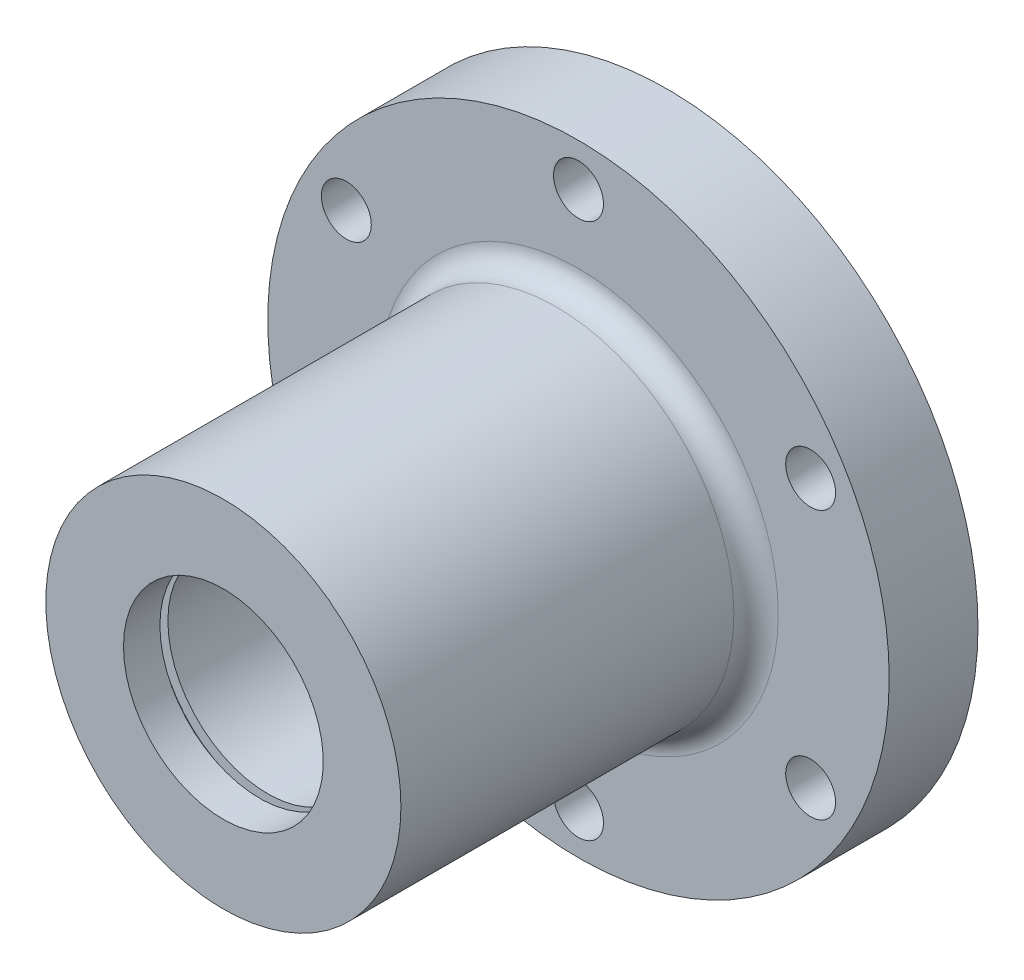
ISO-10303-21;
HEADER;
FILE_DESCRIPTION(('STEP AP214'),'2;1');
FILE_NAME('part.step','',(''),(''),'','','');
FILE_SCHEMA(('AUTOMOTIVE_DESIGN { 1 0 10303 214 1 1 1 1 }'));
ENDSEC;
DATA;
#1=APPLICATION_CONTEXT('core data for automotive mechanical design processes');
#2=APPLICATION_PROTOCOL_DEFINITION('international standard','automotive_design',2000,#1);
#3=PRODUCT_CONTEXT('',#1,'mechanical');
#4=PRODUCT('Part','Part','',(#3));
#5=PRODUCT_RELATED_PRODUCT_CATEGORY('part','',(#4));
#6=PRODUCT_DEFINITION_FORMATION('','',#4);
#7=PRODUCT_DEFINITION_CONTEXT('part definition',#1,'design');
#8=PRODUCT_DEFINITION('design','',#6,#7);
#9=PRODUCT_DEFINITION_SHAPE('','',#8);
#10=(LENGTH_UNIT() NAMED_UNIT(*) SI_UNIT(.MILLI.,.METRE.));
#11=(NAMED_UNIT(*) PLANE_ANGLE_UNIT() SI_UNIT($,.RADIAN.));
#12=(NAMED_UNIT(*) SI_UNIT($,.STERADIAN.) SOLID_ANGLE_UNIT());
#13=UNCERTAINTY_MEASURE_WITH_UNIT(LENGTH_MEASURE(1.E-05),#10,'distance_accuracy_value','');
#14=(GEOMETRIC_REPRESENTATION_CONTEXT(3) GLOBAL_UNCERTAINTY_ASSIGNED_CONTEXT((#13)) GLOBAL_UNIT_ASSIGNED_CONTEXT((#10,
#11,#12)) REPRESENTATION_CONTEXT('',''));
#15=CARTESIAN_POINT('',(0.,0.,0.));
#16=DIRECTION('',(0.,0.,1.));
#17=DIRECTION('',(1.,0.,0.));
#18=AXIS2_PLACEMENT_3D('',#15,#16,#17);
#19=CARTESIAN_POINT('',(0.,0.,12.7));
#20=DIRECTION('',(0.,0.,-1.));
#21=DIRECTION('',(-1.,0.,0.));
#22=AXIS2_PLACEMENT_3D('',#19,#20,#21);
#23=CYLINDRICAL_SURFACE('',#22,44.45);
#24=CARTESIAN_POINT('',(0.,0.,12.7));
#25=DIRECTION('',(0.,0.,1.));
#26=DIRECTION('',(1.,0.,0.));
#27=AXIS2_PLACEMENT_3D('',#24,#25,#26);
#28=CIRCLE('',#27,44.45);
#29=CARTESIAN_POINT('',(44.45,0.,12.7));
#30=VERTEX_POINT('',#29);
#31=EDGE_CURVE('E48',#30,#30,#28,.T.);
#32=ORIENTED_EDGE('',*,*,#31,.F.);
#33=EDGE_LOOP('',(#32));
#34=FACE_BOUND('',#33,.T.);
#35=CARTESIAN_POINT('',(0.,0.,0.));
#36=DIRECTION('',(0.,0.,1.));
#37=DIRECTION('',(1.,0.,0.));
#38=AXIS2_PLACEMENT_3D('',#35,#36,#37);
#39=CIRCLE('',#38,44.45);
#40=CARTESIAN_POINT('',(44.45,0.,0.));
#41=VERTEX_POINT('',#40);
#42=EDGE_CURVE('E55',#41,#41,#39,.T.);
#43=ORIENTED_EDGE('',*,*,#42,.T.);
#44=EDGE_LOOP('',(#43));
#45=FACE_BOUND('',#44,.T.);
#46=ADVANCED_FACE('F40',(#34,#45),#23,.T.);
#47=CARTESIAN_POINT('',(0.,0.,12.7));
#48=DIRECTION('',(0.,0.,1.));
#49=DIRECTION('',(1.,0.,0.));
#50=AXIS2_PLACEMENT_3D('',#47,#48,#49);
#51=PLANE('',#50);
#52=CARTESIAN_POINT('',(0.,0.,12.7));
#53=DIRECTION('',(0.,0.,1.));
#54=DIRECTION('',(1.,0.,0.));
#55=AXIS2_PLACEMENT_3D('',#52,#53,#54);
#56=CIRCLE('',#55,28.575);
#57=CARTESIAN_POINT('',(28.575,0.,12.7));
#58=VERTEX_POINT('',#57);
#59=EDGE_CURVE('E10',#58,#58,#56,.F.);
#60=ORIENTED_EDGE('',*,*,#59,.T.);
#61=EDGE_LOOP('',(#60));
#62=FACE_BOUND('',#61,.T.);
#63=CARTESIAN_POINT('',(-1.25238909962569E-12,38.3450832342934,12.7));
#64=DIRECTION('',(0.,0.,1.));
#65=DIRECTION('',(1.,0.,0.));
#66=AXIS2_PLACEMENT_3D('',#63,#64,#65);
#67=CIRCLE('',#66,3.5687);
#68=CARTESIAN_POINT('',(3.56869999999875,38.3450832342934,12.7));
#69=VERTEX_POINT('',#68);
#70=EDGE_CURVE('E54',#69,#69,#67,.T.);
#71=ORIENTED_EDGE('',*,*,#70,.F.);
#72=EDGE_LOOP('',(#71));
#73=FACE_BOUND('',#72,.T.);
#74=CARTESIAN_POINT('',(33.2078161911255,19.1725416171468,12.7));
#75=DIRECTION('',(0.,0.,1.));
#76=DIRECTION('',(1.,0.,0.));
#77=AXIS2_PLACEMENT_3D('',#74,#75,#76);
#78=CIRCLE('',#77,3.56870000000124);
#79=CARTESIAN_POINT('',(36.7765161911268,19.1725416171468,12.7));
#80=VERTEX_POINT('',#79);
#81=EDGE_CURVE('E56',#80,#80,#78,.T.);
#82=ORIENTED_EDGE('',*,*,#81,.F.);
#83=EDGE_LOOP('',(#82));
#84=FACE_BOUND('',#83,.T.);
#85=CARTESIAN_POINT('',(33.2078161911255,-19.1725416171465,12.7));
#86=DIRECTION('',(0.,0.,1.));
#87=DIRECTION('',(1.,0.,0.));
#88=AXIS2_PLACEMENT_3D('',#85,#86,#87);
#89=CIRCLE('',#88,3.56870000000238);
#90=CARTESIAN_POINT('',(36.7765161911279,-19.1725416171465,12.7));
#91=VERTEX_POINT('',#90);
#92=EDGE_CURVE('E65',#91,#91,#89,.T.);
#93=ORIENTED_EDGE('',*,*,#92,.F.);
#94=EDGE_LOOP('',(#93));
#95=FACE_BOUND('',#94,.T.);
#96=CARTESIAN_POINT('',(-1.20231643282915E-12,-38.3450832342931,12.7));
#97=DIRECTION('',(0.,0.,1.));
#98=DIRECTION('',(1.,0.,0.));
#99=AXIS2_PLACEMENT_3D('',#96,#97,#98);
#100=CIRCLE('',#99,3.56870000000269);
#101=CARTESIAN_POINT('',(3.56870000000149,-38.3450832342931,12.7));
#102=VERTEX_POINT('',#101);
#103=EDGE_CURVE('E61',#102,#102,#100,.T.);
#104=ORIENTED_EDGE('',*,*,#103,.F.);
#105=EDGE_LOOP('',(#104));
#106=FACE_BOUND('',#105,.T.);
#107=CARTESIAN_POINT('',(-33.207816191128,-19.1725416171465,12.7));
#108=DIRECTION('',(0.,0.,1.));
#109=DIRECTION('',(1.,0.,0.));
#110=AXIS2_PLACEMENT_3D('',#107,#108,#109);
#111=CIRCLE('',#110,3.56870000000184);
#112=CARTESIAN_POINT('',(-29.6391161911261,-19.1725416171465,12.7));
#113=VERTEX_POINT('',#112);
#114=EDGE_CURVE('E67',#113,#113,#111,.T.);
#115=ORIENTED_EDGE('',*,*,#114,.F.);
#116=EDGE_LOOP('',(#115));
#117=FACE_BOUND('',#116,.T.);
#118=CARTESIAN_POINT('',(-33.207816191128,19.1725416171468,12.7));
#119=DIRECTION('',(0.,0.,1.));
#120=DIRECTION('',(1.,0.,0.));
#121=AXIS2_PLACEMENT_3D('',#118,#119,#120);
#122=CIRCLE('',#121,3.56870000000052);
#123=CARTESIAN_POINT('',(-29.6391161911275,19.1725416171468,12.7));
#124=VERTEX_POINT('',#123);
#125=EDGE_CURVE('E72',#124,#124,#122,.T.);
#126=ORIENTED_EDGE('',*,*,#125,.F.);
#127=EDGE_LOOP('',(#126));
#128=FACE_BOUND('',#127,.T.);
#129=ORIENTED_EDGE('',*,*,#31,.T.);
#130=EDGE_LOOP('',(#129));
#131=FACE_BOUND('',#130,.T.);
#132=ADVANCED_FACE('F189',(#62,#73,#84,#95,#106,#117,#128,#131),#51,.T.);
#133=CARTESIAN_POINT('',(0.,0.,0.));
#134=DIRECTION('',(0.,0.,1.));
#135=DIRECTION('',(1.,0.,0.));
#136=AXIS2_PLACEMENT_3D('',#133,#134,#135);
#137=PLANE('',#136);
#138=CARTESIAN_POINT('',(-1.25238909962569E-12,38.3450832342934,0.));
#139=DIRECTION('',(0.,0.,-1.));
#140=DIRECTION('',(-1.,0.,0.));
#141=AXIS2_PLACEMENT_3D('',#138,#139,#140);
#142=CIRCLE('',#141,5.15619999999839);
#143=CARTESIAN_POINT('',(-5.15619999999964,38.3450832342934,0.));
#144=VERTEX_POINT('',#143);
#145=EDGE_CURVE('E142',#144,#144,#142,.T.);
#146=ORIENTED_EDGE('',*,*,#145,.F.);
#147=EDGE_LOOP('',(#146));
#148=FACE_BOUND('',#147,.T.);
#149=CARTESIAN_POINT('',(33.2078161911254,19.1725416171464,0.));
#150=DIRECTION('',(0.,0.,-1.));
#151=DIRECTION('',(-1.,0.,0.));
#152=AXIS2_PLACEMENT_3D('',#149,#150,#151);
#153=CIRCLE('',#152,5.1562);
#154=CARTESIAN_POINT('',(28.0516161911254,19.1725416171464,0.));
#155=VERTEX_POINT('',#154);
#156=EDGE_CURVE('E123',#155,#155,#153,.T.);
#157=ORIENTED_EDGE('',*,*,#156,.F.);
#158=EDGE_LOOP('',(#157));
#159=FACE_BOUND('',#158,.T.);
#160=CARTESIAN_POINT('',(33.2078161911251,-19.1725416171471,0.));
#161=DIRECTION('',(0.,0.,-1.));
#162=DIRECTION('',(-1.,0.,0.));
#163=AXIS2_PLACEMENT_3D('',#160,#161,#162);
#164=CIRCLE('',#163,5.15620000000149);
#165=CARTESIAN_POINT('',(28.0516161911236,-19.1725416171471,0.));
#166=VERTEX_POINT('',#165);
#167=EDGE_CURVE('E116',#166,#166,#164,.T.);
#168=ORIENTED_EDGE('',*,*,#167,.F.);
#169=EDGE_LOOP('',(#168));
#170=FACE_BOUND('',#169,.T.);
#171=CARTESIAN_POINT('',(-2.00302158664965E-12,-38.3450832342934,0.));
#172=DIRECTION('',(0.,0.,-1.));
#173=DIRECTION('',(-1.,0.,0.));
#174=AXIS2_PLACEMENT_3D('',#171,#172,#173);
#175=CIRCLE('',#174,5.15620000000176);
#176=CARTESIAN_POINT('',(-5.15620000000376,-38.3450832342934,0.));
#177=VERTEX_POINT('',#176);
#178=EDGE_CURVE('E130',#177,#177,#175,.T.);
#179=ORIENTED_EDGE('',*,*,#178,.F.);
#180=EDGE_LOOP('',(#179));
#181=FACE_BOUND('',#180,.T.);
#182=CARTESIAN_POINT('',(-33.2078161911287,-19.1725416171464,0.));
#183=DIRECTION('',(0.,0.,-1.));
#184=DIRECTION('',(-1.,0.,0.));
#185=AXIS2_PLACEMENT_3D('',#182,#183,#184);
#186=CIRCLE('',#185,5.15620000000049);
#187=CARTESIAN_POINT('',(-38.3640161911292,-19.1725416171464,0.));
#188=VERTEX_POINT('',#187);
#189=EDGE_CURVE('E133',#188,#188,#186,.T.);
#190=ORIENTED_EDGE('',*,*,#189,.F.);
#191=EDGE_LOOP('',(#190));
#192=FACE_BOUND('',#191,.T.);
#193=CARTESIAN_POINT('',(-33.2078161911283,19.172541617147,0.));
#194=DIRECTION('',(0.,0.,-1.));
#195=DIRECTION('',(-1.,0.,0.));
#196=AXIS2_PLACEMENT_3D('',#193,#194,#195);
#197=CIRCLE('',#196,5.15619999999885);
#198=CARTESIAN_POINT('',(-38.3640161911271,19.172541617147,0.));
#199=VERTEX_POINT('',#198);
#200=EDGE_CURVE('E140',#199,#199,#197,.T.);
#201=ORIENTED_EDGE('',*,*,#200,.F.);
#202=EDGE_LOOP('',(#201));
#203=FACE_BOUND('',#202,.T.);
#204=CARTESIAN_POINT('',(0.,0.,0.));
#205=DIRECTION('',(0.,0.,-1.));
#206=DIRECTION('',(-1.,0.,0.));
#207=AXIS2_PLACEMENT_3D('',#204,#205,#206);
#208=CIRCLE('',#207,20.6375);
#209=CARTESIAN_POINT('',(-20.6375,0.,0.));
#210=VERTEX_POINT('',#209);
#211=EDGE_CURVE('E83',#210,#210,#208,.T.);
#212=ORIENTED_EDGE('',*,*,#211,.F.);
#213=EDGE_LOOP('',(#212));
#214=FACE_BOUND('',#213,.T.);
#215=ORIENTED_EDGE('',*,*,#42,.F.);
#216=EDGE_LOOP('',(#215));
#217=FACE_BOUND('',#216,.T.);
#218=ADVANCED_FACE('F183',(#148,#159,#170,#181,#192,#203,#214,#217),#137,.F.);
#219=CARTESIAN_POINT('',(0.,0.,63.5));
#220=DIRECTION('',(0.,0.,-1.));
#221=DIRECTION('',(-1.,0.,0.));
#222=AXIS2_PLACEMENT_3D('',#219,#220,#221);
#223=CYLINDRICAL_SURFACE('',#222,25.4);
#224=CARTESIAN_POINT('',(0.,0.,15.875));
#225=DIRECTION('',(0.,0.,1.));
#226=DIRECTION('',(1.,0.,0.));
#227=AXIS2_PLACEMENT_3D('',#224,#225,#226);
#228=CIRCLE('',#227,25.4);
#229=CARTESIAN_POINT('',(25.4,0.,15.875));
#230=VERTEX_POINT('',#229);
#231=EDGE_CURVE('E42',#230,#230,#228,.T.);
#232=ORIENTED_EDGE('',*,*,#231,.T.);
#233=EDGE_LOOP('',(#232));
#234=FACE_BOUND('',#233,.T.);
#235=CARTESIAN_POINT('',(0.,0.,63.5));
#236=DIRECTION('',(0.,0.,1.));
#237=DIRECTION('',(1.,0.,0.));
#238=AXIS2_PLACEMENT_3D('',#235,#236,#237);
#239=CIRCLE('',#238,25.4);
#240=CARTESIAN_POINT('',(25.4,0.,63.5));
#241=VERTEX_POINT('',#240);
#242=EDGE_CURVE('E77',#241,#241,#239,.T.);
#243=ORIENTED_EDGE('',*,*,#242,.F.);
#244=EDGE_LOOP('',(#243));
#245=FACE_BOUND('',#244,.T.);
#246=ADVANCED_FACE('F188',(#234,#245),#223,.T.);
#247=CARTESIAN_POINT('',(0.,0.,63.5));
#248=DIRECTION('',(0.,0.,1.));
#249=DIRECTION('',(1.,0.,0.));
#250=AXIS2_PLACEMENT_3D('',#247,#248,#249);
#251=PLANE('',#250);
#252=CARTESIAN_POINT('',(0.,0.,63.5));
#253=DIRECTION('',(0.,0.,-1.));
#254=DIRECTION('',(-1.,0.,0.));
#255=AXIS2_PLACEMENT_3D('',#252,#253,#254);
#256=CIRCLE('',#255,14.2875);
#257=CARTESIAN_POINT('',(-14.2875,0.,63.5));
#258=VERTEX_POINT('',#257);
#259=EDGE_CURVE('E107',#258,#258,#256,.T.);
#260=ORIENTED_EDGE('',*,*,#259,.T.);
#261=EDGE_LOOP('',(#260));
#262=FACE_BOUND('',#261,.T.);
#263=ORIENTED_EDGE('',*,*,#242,.T.);
#264=EDGE_LOOP('',(#263));
#265=FACE_BOUND('',#264,.T.);
#266=ADVANCED_FACE('F216',(#262,#265),#251,.T.);
#267=CARTESIAN_POINT('',(0.,0.,6.35));
#268=DIRECTION('',(0.,0.,-1.));
#269=DIRECTION('',(-1.,0.,0.));
#270=AXIS2_PLACEMENT_3D('',#267,#268,#269);
#271=CYLINDRICAL_SURFACE('',#270,20.6375);
#272=CARTESIAN_POINT('',(0.,0.,6.35));
#273=DIRECTION('',(0.,0.,-1.));
#274=DIRECTION('',(-1.,0.,0.));
#275=AXIS2_PLACEMENT_3D('',#272,#273,#274);
#276=CIRCLE('',#275,20.6375);
#277=CARTESIAN_POINT('',(-20.6375,0.,6.35));
#278=VERTEX_POINT('',#277);
#279=EDGE_CURVE('E76',#278,#278,#276,.T.);
#280=ORIENTED_EDGE('',*,*,#279,.F.);
#281=EDGE_LOOP('',(#280));
#282=FACE_BOUND('',#281,.T.);
#283=ORIENTED_EDGE('',*,*,#211,.T.);
#284=EDGE_LOOP('',(#283));
#285=FACE_BOUND('',#284,.T.);
#286=ADVANCED_FACE('F218',(#282,#285),#271,.F.);
#287=CARTESIAN_POINT('',(0.,0.,6.35));
#288=DIRECTION('',(0.,0.,-1.));
#289=DIRECTION('',(-1.,0.,0.));
#290=AXIS2_PLACEMENT_3D('',#287,#288,#289);
#291=PLANE('',#290);
#292=CARTESIAN_POINT('',(0.,0.,6.35));
#293=DIRECTION('',(0.,0.,-1.));
#294=DIRECTION('',(-1.,0.,0.));
#295=AXIS2_PLACEMENT_3D('',#292,#293,#294);
#296=CIRCLE('',#295,9.525);
#297=CARTESIAN_POINT('',(-9.525,0.,6.35));
#298=VERTEX_POINT('',#297);
#299=EDGE_CURVE('E85',#298,#298,#296,.T.);
#300=ORIENTED_EDGE('',*,*,#299,.F.);
#301=EDGE_LOOP('',(#300));
#302=FACE_BOUND('',#301,.T.);
#303=ORIENTED_EDGE('',*,*,#279,.T.);
#304=EDGE_LOOP('',(#303));
#305=FACE_BOUND('',#304,.T.);
#306=ADVANCED_FACE('F225',(#302,#305),#291,.T.);
#307=CARTESIAN_POINT('',(0.,0.,15.875));
#308=DIRECTION('',(0.,0.,-1.));
#309=DIRECTION('',(-1.,0.,0.));
#310=AXIS2_PLACEMENT_3D('',#307,#308,#309);
#311=CYLINDRICAL_SURFACE('',#310,9.525);
#312=CARTESIAN_POINT('',(0.,0.,15.875));
#313=DIRECTION('',(0.,0.,-1.));
#314=DIRECTION('',(-1.,0.,0.));
#315=AXIS2_PLACEMENT_3D('',#312,#313,#314);
#316=CIRCLE('',#315,9.525);
#317=CARTESIAN_POINT('',(-9.525,0.,15.875));
#318=VERTEX_POINT('',#317);
#319=EDGE_CURVE('E90',#318,#318,#316,.T.);
#320=CARTESIAN_POINT('',(-9.525,0.,15.875));
#321=CARTESIAN_POINT('',(-9.525,0.,15.77578125));
#322=CARTESIAN_POINT('',(-9.525,0.,15.6765625));
#323=CARTESIAN_POINT('',(-9.525,0.,15.478125));
#324=CARTESIAN_POINT('',(-9.525,0.,15.37890625));
#325=CARTESIAN_POINT('',(-9.525,0.,15.18046875));
#326=CARTESIAN_POINT('',(-9.525,0.,15.08125));
#327=CARTESIAN_POINT('',(-9.525,0.,14.8828125));
#328=CARTESIAN_POINT('',(-9.525,0.,14.78359375));
#329=CARTESIAN_POINT('',(-9.525,0.,14.58515625));
#330=CARTESIAN_POINT('',(-9.525,0.,14.4859375));
#331=CARTESIAN_POINT('',(-9.525,0.,14.2875));
#332=CARTESIAN_POINT('',(-9.525,0.,14.18828125));
#333=CARTESIAN_POINT('',(-9.525,0.,13.98984375));
#334=CARTESIAN_POINT('',(-9.525,0.,13.890625));
#335=CARTESIAN_POINT('',(-9.525,0.,13.6921875));
#336=CARTESIAN_POINT('',(-9.525,0.,13.59296875));
#337=CARTESIAN_POINT('',(-9.525,0.,13.39453125));
#338=CARTESIAN_POINT('',(-9.525,0.,13.2953125));
#339=CARTESIAN_POINT('',(-9.525,0.,13.096875));
#340=CARTESIAN_POINT('',(-9.525,0.,12.99765625));
#341=CARTESIAN_POINT('',(-9.525,0.,12.79921875));
#342=CARTESIAN_POINT('',(-9.525,0.,12.7));
#343=CARTESIAN_POINT('',(-9.525,0.,12.5015625));
#344=CARTESIAN_POINT('',(-9.525,0.,12.40234375));
#345=CARTESIAN_POINT('',(-9.525,0.,12.20390625));
#346=CARTESIAN_POINT('',(-9.525,0.,12.1046875));
#347=CARTESIAN_POINT('',(-9.525,0.,11.90625));
#348=CARTESIAN_POINT('',(-9.525,0.,11.80703125));
#349=CARTESIAN_POINT('',(-9.525,0.,11.60859375));
#350=CARTESIAN_POINT('',(-9.525,0.,11.509375));
#351=CARTESIAN_POINT('',(-9.525,0.,11.3109375));
#352=CARTESIAN_POINT('',(-9.525,0.,11.21171875));
#353=CARTESIAN_POINT('',(-9.525,0.,11.01328125));
#354=CARTESIAN_POINT('',(-9.525,0.,10.9140625));
#355=CARTESIAN_POINT('',(-9.525,0.,10.715625));
#356=CARTESIAN_POINT('',(-9.525,0.,10.61640625));
#357=CARTESIAN_POINT('',(-9.525,0.,10.41796875));
#358=CARTESIAN_POINT('',(-9.525,0.,10.31875));
#359=CARTESIAN_POINT('',(-9.525,0.,10.1203125));
#360=CARTESIAN_POINT('',(-9.525,0.,10.02109375));
#361=CARTESIAN_POINT('',(-9.525,0.,9.82265625));
#362=CARTESIAN_POINT('',(-9.525,0.,9.7234375));
#363=CARTESIAN_POINT('',(-9.525,0.,9.525));
#364=CARTESIAN_POINT('',(-9.525,0.,9.42578125));
#365=CARTESIAN_POINT('',(-9.525,0.,9.22734375));
#366=CARTESIAN_POINT('',(-9.525,0.,9.128125));
#367=CARTESIAN_POINT('',(-9.525,0.,8.9296875));
#368=CARTESIAN_POINT('',(-9.525,0.,8.83046875));
#369=CARTESIAN_POINT('',(-9.525,0.,8.63203125));
#370=CARTESIAN_POINT('',(-9.525,0.,8.5328125));
#371=CARTESIAN_POINT('',(-9.525,0.,8.334375));
#372=CARTESIAN_POINT('',(-9.525,0.,8.23515625));
#373=CARTESIAN_POINT('',(-9.525,0.,8.03671875));
#374=CARTESIAN_POINT('',(-9.525,0.,7.9375));
#375=CARTESIAN_POINT('',(-9.525,0.,7.7390625));
#376=CARTESIAN_POINT('',(-9.525,0.,7.63984375));
#377=CARTESIAN_POINT('',(-9.525,0.,7.44140625));
#378=CARTESIAN_POINT('',(-9.525,0.,7.3421875));
#379=CARTESIAN_POINT('',(-9.525,0.,7.14375));
#380=CARTESIAN_POINT('',(-9.525,0.,7.04453125));
#381=CARTESIAN_POINT('',(-9.525,0.,6.84609375));
#382=CARTESIAN_POINT('',(-9.525,0.,6.746875));
#383=CARTESIAN_POINT('',(-9.525,0.,6.5484375));
#384=CARTESIAN_POINT('',(-9.525,0.,6.44921875));
#385=CARTESIAN_POINT('',(-9.525,0.,6.35));
#386=B_SPLINE_CURVE_WITH_KNOTS('',3,(#320,#321,#322,#323,#324,#325,#326,#327,#328,#329,#330,
#331,#332,#333,#334,#335,#336,#337,#338,#339,#340,#341,#342,#343,#344,#345,#346,#347,#348,#349,
#350,#351,#352,#353,#354,#355,#356,#357,#358,#359,#360,#361,#362,#363,#364,#365,#366,#367,#368,
#369,#370,#371,#372,#373,#374,#375,#376,#377,#378,#379,#380,#381,#382,#383,#384,#385),
.UNSPECIFIED.,.F.,.F.,(4,2,2,2,2,2,2,2,2,2,2,2,2,2,2,2,2,2,2,2,2,2,2,2,2,2,2,2,2,2,2,2,4),(0.,
0.297656249999998,0.595312499999999,0.892968749999999,1.190625,1.48828125,1.7859375,2.08359375,
2.38125,2.67890625,2.9765625,3.27421875,3.571875,3.86953125,4.1671875,4.46484375,4.7625,
5.06015625,5.3578125,5.65546875,5.953125,6.25078125,6.5484375,6.84609375,7.14375,7.44140625,
7.7390625,8.03671875,8.334375,8.63203125,8.9296875,9.22734375,9.525),.UNSPECIFIED.);
#387=EDGE_CURVE('BSEAM227',#318,#298,#386,.T.);
#388=ORIENTED_EDGE('',*,*,#319,.F.);
#389=ORIENTED_EDGE('',*,*,#299,.T.);
#390=ORIENTED_EDGE('',*,*,#387,.T.);
#391=ORIENTED_EDGE('',*,*,#387,.F.);
#392=EDGE_LOOP('',(#388,#390,#389,#391));
#393=FACE_BOUND('',#392,.T.);
#394=ADVANCED_FACE('F227',(#393),#311,.F.);
#395=CARTESIAN_POINT('',(0.,0.,41.275));
#396=DIRECTION('',(0.,0.,-1.));
#397=DIRECTION('',(-1.,0.,0.));
#398=AXIS2_PLACEMENT_3D('',#395,#396,#397);
#399=CYLINDRICAL_SURFACE('',#398,12.7);
#400=CARTESIAN_POINT('',(0.,0.,41.275));
#401=DIRECTION('',(0.,0.,-1.));
#402=DIRECTION('',(-1.,0.,0.));
#403=AXIS2_PLACEMENT_3D('',#400,#401,#402);
#404=CIRCLE('',#403,12.7);
#405=CARTESIAN_POINT('',(-12.7,0.,41.275));
#406=VERTEX_POINT('',#405);
#407=EDGE_CURVE('E92',#406,#406,#404,.T.);
#408=ORIENTED_EDGE('',*,*,#407,.F.);
#409=EDGE_LOOP('',(#408));
#410=FACE_BOUND('',#409,.T.);
#411=CARTESIAN_POINT('',(0.,0.,15.875));
#412=DIRECTION('',(0.,0.,-1.));
#413=DIRECTION('',(-1.,0.,0.));
#414=AXIS2_PLACEMENT_3D('',#411,#412,#413);
#415=CIRCLE('',#414,12.7);
#416=CARTESIAN_POINT('',(-12.7,0.,15.875));
#417=VERTEX_POINT('',#416);
#418=EDGE_CURVE('E95',#417,#417,#415,.T.);
#419=ORIENTED_EDGE('',*,*,#418,.T.);
#420=EDGE_LOOP('',(#419));
#421=FACE_BOUND('',#420,.T.);
#422=ADVANCED_FACE('F226',(#410,#421),#399,.F.);
#423=CARTESIAN_POINT('',(0.,0.,15.875));
#424=DIRECTION('',(0.,0.,-1.));
#425=DIRECTION('',(-1.,0.,0.));
#426=AXIS2_PLACEMENT_3D('',#423,#424,#425);
#427=PLANE('',#426);
#428=ORIENTED_EDGE('',*,*,#319,.T.);
#429=EDGE_LOOP('',(#428));
#430=FACE_BOUND('',#429,.T.);
#431=ORIENTED_EDGE('',*,*,#418,.F.);
#432=EDGE_LOOP('',(#431));
#433=FACE_BOUND('',#432,.T.);
#434=ADVANCED_FACE('F235',(#430,#433),#427,.F.);
#435=CARTESIAN_POINT('',(0.,0.,57.15));
#436=DIRECTION('',(0.,0.,-1.));
#437=DIRECTION('',(-1.,0.,0.));
#438=AXIS2_PLACEMENT_3D('',#435,#436,#437);
#439=CYLINDRICAL_SURFACE('',#438,14.2875);
#440=CARTESIAN_POINT('',(0.,0.,57.15));
#441=DIRECTION('',(0.,0.,-1.));
#442=DIRECTION('',(-1.,0.,0.));
#443=AXIS2_PLACEMENT_3D('',#440,#441,#442);
#444=CIRCLE('',#443,14.2875);
#445=CARTESIAN_POINT('',(-14.2875,0.,57.15));
#446=VERTEX_POINT('',#445);
#447=EDGE_CURVE('E101',#446,#446,#444,.T.);
#448=ORIENTED_EDGE('',*,*,#447,.F.);
#449=EDGE_LOOP('',(#448));
#450=FACE_BOUND('',#449,.T.);
#451=CARTESIAN_POINT('',(0.,0.,41.275));
#452=DIRECTION('',(0.,0.,-1.));
#453=DIRECTION('',(-1.,0.,0.));
#454=AXIS2_PLACEMENT_3D('',#451,#452,#453);
#455=CIRCLE('',#454,14.2875);
#456=CARTESIAN_POINT('',(-14.2875,0.,41.275));
#457=VERTEX_POINT('',#456);
#458=EDGE_CURVE('E98',#457,#457,#455,.T.);
#459=ORIENTED_EDGE('',*,*,#458,.T.);
#460=EDGE_LOOP('',(#459));
#461=FACE_BOUND('',#460,.T.);
#462=ADVANCED_FACE('F236',(#450,#461),#439,.F.);
#463=CARTESIAN_POINT('',(0.,0.,41.275));
#464=DIRECTION('',(0.,0.,-1.));
#465=DIRECTION('',(-1.,0.,0.));
#466=AXIS2_PLACEMENT_3D('',#463,#464,#465);
#467=PLANE('',#466);
#468=ORIENTED_EDGE('',*,*,#407,.T.);
#469=EDGE_LOOP('',(#468));
#470=FACE_BOUND('',#469,.T.);
#471=ORIENTED_EDGE('',*,*,#458,.F.);
#472=EDGE_LOOP('',(#471));
#473=FACE_BOUND('',#472,.T.);
#474=ADVANCED_FACE('F245',(#470,#473),#467,.F.);
#475=CARTESIAN_POINT('',(0.,0.,58.293));
#476=DIRECTION('',(0.,0.,-1.));
#477=DIRECTION('',(-1.,0.,0.));
#478=AXIS2_PLACEMENT_3D('',#475,#476,#477);
#479=CYLINDRICAL_SURFACE('',#478,15.8115);
#480=CARTESIAN_POINT('',(0.,0.,58.293));
#481=DIRECTION('',(0.,0.,-1.));
#482=DIRECTION('',(-1.,0.,0.));
#483=AXIS2_PLACEMENT_3D('',#480,#481,#482);
#484=CIRCLE('',#483,15.8115);
#485=CARTESIAN_POINT('',(-15.8115,0.,58.293));
#486=VERTEX_POINT('',#485);
#487=EDGE_CURVE('E102',#486,#486,#484,.T.);
#488=ORIENTED_EDGE('',*,*,#487,.F.);
#489=EDGE_LOOP('',(#488));
#490=FACE_BOUND('',#489,.T.);
#491=CARTESIAN_POINT('',(0.,0.,57.15));
#492=DIRECTION('',(0.,0.,-1.));
#493=DIRECTION('',(-1.,0.,0.));
#494=AXIS2_PLACEMENT_3D('',#491,#492,#493);
#495=CIRCLE('',#494,15.8115);
#496=CARTESIAN_POINT('',(-15.8115,0.,57.15));
#497=VERTEX_POINT('',#496);
#498=EDGE_CURVE('E104',#497,#497,#495,.T.);
#499=ORIENTED_EDGE('',*,*,#498,.T.);
#500=EDGE_LOOP('',(#499));
#501=FACE_BOUND('',#500,.T.);
#502=ADVANCED_FACE('F248',(#490,#501),#479,.F.);
#503=CARTESIAN_POINT('',(0.,0.,58.293));
#504=DIRECTION('',(0.,0.,-1.));
#505=DIRECTION('',(-1.,0.,0.));
#506=AXIS2_PLACEMENT_3D('',#503,#504,#505);
#507=PLANE('',#506);
#508=CARTESIAN_POINT('',(0.,0.,58.293));
#509=DIRECTION('',(0.,0.,-1.));
#510=DIRECTION('',(-1.,0.,0.));
#511=AXIS2_PLACEMENT_3D('',#508,#509,#510);
#512=CIRCLE('',#511,14.2875);
#513=CARTESIAN_POINT('',(-14.2875,0.,58.293));
#514=VERTEX_POINT('',#513);
#515=EDGE_CURVE('E112',#514,#514,#512,.T.);
#516=ORIENTED_EDGE('',*,*,#515,.F.);
#517=EDGE_LOOP('',(#516));
#518=FACE_BOUND('',#517,.T.);
#519=ORIENTED_EDGE('',*,*,#487,.T.);
#520=EDGE_LOOP('',(#519));
#521=FACE_BOUND('',#520,.T.);
#522=ADVANCED_FACE('F246',(#518,#521),#507,.T.);
#523=CARTESIAN_POINT('',(0.,0.,57.15));
#524=DIRECTION('',(0.,0.,-1.));
#525=DIRECTION('',(-1.,0.,0.));
#526=AXIS2_PLACEMENT_3D('',#523,#524,#525);
#527=PLANE('',#526);
#528=ORIENTED_EDGE('',*,*,#447,.T.);
#529=EDGE_LOOP('',(#528));
#530=FACE_BOUND('',#529,.T.);
#531=ORIENTED_EDGE('',*,*,#498,.F.);
#532=EDGE_LOOP('',(#531));
#533=FACE_BOUND('',#532,.T.);
#534=ADVANCED_FACE('F252',(#530,#533),#527,.F.);
#535=CARTESIAN_POINT('',(0.,0.,63.5));
#536=DIRECTION('',(0.,0.,-1.));
#537=DIRECTION('',(-1.,0.,0.));
#538=AXIS2_PLACEMENT_3D('',#535,#536,#537);
#539=CYLINDRICAL_SURFACE('',#538,14.2875);
#540=ORIENTED_EDGE('',*,*,#259,.F.);
#541=EDGE_LOOP('',(#540));
#542=FACE_BOUND('',#541,.T.);
#543=ORIENTED_EDGE('',*,*,#515,.T.);
#544=EDGE_LOOP('',(#543));
#545=FACE_BOUND('',#544,.T.);
#546=ADVANCED_FACE('F254',(#542,#545),#539,.F.);
#547=CARTESIAN_POINT('',(-33.2078161911283,19.172541617147,6.35));
#548=DIRECTION('',(0.,0.,-1.));
#549=DIRECTION('',(-1.,0.,0.));
#550=AXIS2_PLACEMENT_3D('',#547,#548,#549);
#551=CYLINDRICAL_SURFACE('',#550,5.15619999999885);
#552=CARTESIAN_POINT('',(-33.2078161911283,19.172541617147,6.35));
#553=DIRECTION('',(0.,0.,-1.));
#554=DIRECTION('',(-1.,0.,0.));
#555=AXIS2_PLACEMENT_3D('',#552,#553,#554);
#556=CIRCLE('',#555,5.15619999999885);
#557=CARTESIAN_POINT('',(-38.3640161911271,19.172541617147,6.35));
#558=VERTEX_POINT('',#557);
#559=EDGE_CURVE('E138',#558,#558,#556,.T.);
#560=ORIENTED_EDGE('',*,*,#559,.F.);
#561=EDGE_LOOP('',(#560));
#562=FACE_BOUND('',#561,.T.);
#563=ORIENTED_EDGE('',*,*,#200,.T.);
#564=EDGE_LOOP('',(#563));
#565=FACE_BOUND('',#564,.T.);
#566=ADVANCED_FACE('F265',(#562,#565),#551,.F.);
#567=CARTESIAN_POINT('',(-33.2078161911283,19.172541617147,6.35));
#568=DIRECTION('',(0.,0.,-1.));
#569=DIRECTION('',(-1.,0.,0.));
#570=AXIS2_PLACEMENT_3D('',#567,#568,#569);
#571=PLANE('',#570);
#572=CARTESIAN_POINT('',(-33.207816191128,19.1725416171468,6.35));
#573=DIRECTION('',(0.,0.,-1.));
#574=DIRECTION('',(-1.,0.,0.));
#575=AXIS2_PLACEMENT_3D('',#572,#573,#574);
#576=CIRCLE('',#575,3.56870000000052);
#577=CARTESIAN_POINT('',(-36.7765161911285,19.1725416171468,6.35));
#578=VERTEX_POINT('',#577);
#579=EDGE_CURVE('E161',#578,#578,#576,.T.);
#580=ORIENTED_EDGE('',*,*,#579,.F.);
#581=EDGE_LOOP('',(#580));
#582=FACE_BOUND('',#581,.T.);
#583=ORIENTED_EDGE('',*,*,#559,.T.);
#584=EDGE_LOOP('',(#583));
#585=FACE_BOUND('',#584,.T.);
#586=ADVANCED_FACE('F287',(#582,#585),#571,.T.);
#587=CARTESIAN_POINT('',(-33.2078161911287,-19.1725416171464,6.35));
#588=DIRECTION('',(0.,0.,-1.));
#589=DIRECTION('',(-1.,0.,0.));
#590=AXIS2_PLACEMENT_3D('',#587,#588,#589);
#591=CYLINDRICAL_SURFACE('',#590,5.15620000000049);
#592=CARTESIAN_POINT('',(-33.2078161911287,-19.1725416171464,6.35));
#593=DIRECTION('',(0.,0.,-1.));
#594=DIRECTION('',(-1.,0.,0.));
#595=AXIS2_PLACEMENT_3D('',#592,#593,#594);
#596=CIRCLE('',#595,5.15620000000049);
#597=CARTESIAN_POINT('',(-38.3640161911292,-19.1725416171464,6.35));
#598=VERTEX_POINT('',#597);
#599=EDGE_CURVE('E128',#598,#598,#596,.T.);
#600=ORIENTED_EDGE('',*,*,#599,.F.);
#601=EDGE_LOOP('',(#600));
#602=FACE_BOUND('',#601,.T.);
#603=ORIENTED_EDGE('',*,*,#189,.T.);
#604=EDGE_LOOP('',(#603));
#605=FACE_BOUND('',#604,.T.);
#606=ADVANCED_FACE('F284',(#602,#605),#591,.F.);
#607=CARTESIAN_POINT('',(-33.2078161911287,-19.1725416171464,6.35));
#608=DIRECTION('',(0.,0.,-1.));
#609=DIRECTION('',(-1.,0.,0.));
#610=AXIS2_PLACEMENT_3D('',#607,#608,#609);
#611=PLANE('',#610);
#612=CARTESIAN_POINT('',(-33.207816191128,-19.1725416171465,6.35));
#613=DIRECTION('',(0.,0.,-1.));
#614=DIRECTION('',(-1.,0.,0.));
#615=AXIS2_PLACEMENT_3D('',#612,#613,#614);
#616=CIRCLE('',#615,3.56870000000184);
#617=CARTESIAN_POINT('',(-36.7765161911298,-19.1725416171465,6.35));
#618=VERTEX_POINT('',#617);
#619=EDGE_CURVE('E158',#618,#618,#616,.T.);
#620=ORIENTED_EDGE('',*,*,#619,.F.);
#621=EDGE_LOOP('',(#620));
#622=FACE_BOUND('',#621,.T.);
#623=ORIENTED_EDGE('',*,*,#599,.T.);
#624=EDGE_LOOP('',(#623));
#625=FACE_BOUND('',#624,.T.);
#626=ADVANCED_FACE('F278',(#622,#625),#611,.T.);
#627=CARTESIAN_POINT('',(-2.00302158664965E-12,-38.3450832342934,6.35));
#628=DIRECTION('',(0.,0.,-1.));
#629=DIRECTION('',(-1.,0.,0.));
#630=AXIS2_PLACEMENT_3D('',#627,#628,#629);
#631=CYLINDRICAL_SURFACE('',#630,5.15620000000176);
#632=CARTESIAN_POINT('',(-2.00302158664965E-12,-38.3450832342934,6.35));
#633=DIRECTION('',(0.,0.,-1.));
#634=DIRECTION('',(-1.,0.,0.));
#635=AXIS2_PLACEMENT_3D('',#632,#633,#634);
#636=CIRCLE('',#635,5.15620000000176);
#637=CARTESIAN_POINT('',(-5.15620000000376,-38.3450832342934,6.35));
#638=VERTEX_POINT('',#637);
#639=EDGE_CURVE('E125',#638,#638,#636,.T.);
#640=ORIENTED_EDGE('',*,*,#639,.F.);
#641=EDGE_LOOP('',(#640));
#642=FACE_BOUND('',#641,.T.);
#643=ORIENTED_EDGE('',*,*,#178,.T.);
#644=EDGE_LOOP('',(#643));
#645=FACE_BOUND('',#644,.T.);
#646=ADVANCED_FACE('F277',(#642,#645),#631,.F.);
#647=CARTESIAN_POINT('',(-2.00302158664965E-12,-38.3450832342934,6.35));
#648=DIRECTION('',(0.,0.,-1.));
#649=DIRECTION('',(-1.,0.,0.));
#650=AXIS2_PLACEMENT_3D('',#647,#648,#649);
#651=PLANE('',#650);
#652=CARTESIAN_POINT('',(-1.20231643282915E-12,-38.3450832342931,6.35));
#653=DIRECTION('',(0.,0.,-1.));
#654=DIRECTION('',(-1.,0.,0.));
#655=AXIS2_PLACEMENT_3D('',#652,#653,#654);
#656=CIRCLE('',#655,3.56870000000269);
#657=CARTESIAN_POINT('',(-3.56870000000389,-38.3450832342931,6.35));
#658=VERTEX_POINT('',#657);
#659=EDGE_CURVE('E152',#658,#658,#656,.T.);
#660=ORIENTED_EDGE('',*,*,#659,.F.);
#661=EDGE_LOOP('',(#660));
#662=FACE_BOUND('',#661,.T.);
#663=ORIENTED_EDGE('',*,*,#639,.T.);
#664=EDGE_LOOP('',(#663));
#665=FACE_BOUND('',#664,.T.);
#666=ADVANCED_FACE('F275',(#662,#665),#651,.T.);
#667=CARTESIAN_POINT('',(33.2078161911251,-19.1725416171471,6.35));
#668=DIRECTION('',(0.,0.,-1.));
#669=DIRECTION('',(-1.,0.,0.));
#670=AXIS2_PLACEMENT_3D('',#667,#668,#669);
#671=CYLINDRICAL_SURFACE('',#670,5.15620000000149);
#672=CARTESIAN_POINT('',(33.2078161911251,-19.1725416171471,6.35));
#673=DIRECTION('',(0.,0.,-1.));
#674=DIRECTION('',(-1.,0.,0.));
#675=AXIS2_PLACEMENT_3D('',#672,#673,#674);
#676=CIRCLE('',#675,5.15620000000149);
#677=CARTESIAN_POINT('',(28.0516161911236,-19.1725416171471,6.35));
#678=VERTEX_POINT('',#677);
#679=EDGE_CURVE('E120',#678,#678,#676,.T.);
#680=ORIENTED_EDGE('',*,*,#679,.F.);
#681=EDGE_LOOP('',(#680));
#682=FACE_BOUND('',#681,.T.);
#683=ORIENTED_EDGE('',*,*,#167,.T.);
#684=EDGE_LOOP('',(#683));
#685=FACE_BOUND('',#684,.T.);
#686=ADVANCED_FACE('F268',(#682,#685),#671,.F.);
#687=CARTESIAN_POINT('',(33.2078161911251,-19.1725416171471,6.35));
#688=DIRECTION('',(0.,0.,-1.));
#689=DIRECTION('',(-1.,0.,0.));
#690=AXIS2_PLACEMENT_3D('',#687,#688,#689);
#691=PLANE('',#690);
#692=CARTESIAN_POINT('',(33.2078161911255,-19.1725416171465,6.35));
#693=DIRECTION('',(0.,0.,-1.));
#694=DIRECTION('',(-1.,0.,0.));
#695=AXIS2_PLACEMENT_3D('',#692,#693,#694);
#696=CIRCLE('',#695,3.56870000000238);
#697=CARTESIAN_POINT('',(29.6391161911231,-19.1725416171465,6.35));
#698=VERTEX_POINT('',#697);
#699=EDGE_CURVE('E151',#698,#698,#696,.T.);
#700=ORIENTED_EDGE('',*,*,#699,.F.);
#701=EDGE_LOOP('',(#700));
#702=FACE_BOUND('',#701,.T.);
#703=ORIENTED_EDGE('',*,*,#679,.T.);
#704=EDGE_LOOP('',(#703));
#705=FACE_BOUND('',#704,.T.);
#706=ADVANCED_FACE('F262',(#702,#705),#691,.T.);
#707=CARTESIAN_POINT('',(33.2078161911254,19.1725416171464,6.35));
#708=DIRECTION('',(0.,0.,-1.));
#709=DIRECTION('',(-1.,0.,0.));
#710=AXIS2_PLACEMENT_3D('',#707,#708,#709);
#711=CYLINDRICAL_SURFACE('',#710,5.1562);
#712=CARTESIAN_POINT('',(33.2078161911254,19.1725416171464,6.35));
#713=DIRECTION('',(0.,0.,-1.));
#714=DIRECTION('',(-1.,0.,0.));
#715=AXIS2_PLACEMENT_3D('',#712,#713,#714);
#716=CIRCLE('',#715,5.1562);
#717=CARTESIAN_POINT('',(28.0516161911254,19.1725416171464,6.35));
#718=VERTEX_POINT('',#717);
#719=EDGE_CURVE('E59',#718,#718,#716,.T.);
#720=ORIENTED_EDGE('',*,*,#719,.F.);
#721=EDGE_LOOP('',(#720));
#722=FACE_BOUND('',#721,.T.);
#723=ORIENTED_EDGE('',*,*,#156,.T.);
#724=EDGE_LOOP('',(#723));
#725=FACE_BOUND('',#724,.T.);
#726=ADVANCED_FACE('F270',(#722,#725),#711,.F.);
#727=CARTESIAN_POINT('',(33.2078161911254,19.1725416171464,6.35));
#728=DIRECTION('',(0.,0.,-1.));
#729=DIRECTION('',(-1.,0.,0.));
#730=AXIS2_PLACEMENT_3D('',#727,#728,#729);
#731=PLANE('',#730);
#732=CARTESIAN_POINT('',(33.2078161911255,19.1725416171468,6.35));
#733=DIRECTION('',(0.,0.,-1.));
#734=DIRECTION('',(-1.,0.,0.));
#735=AXIS2_PLACEMENT_3D('',#732,#733,#734);
#736=CIRCLE('',#735,3.56870000000124);
#737=CARTESIAN_POINT('',(29.6391161911243,19.1725416171468,6.35));
#738=VERTEX_POINT('',#737);
#739=EDGE_CURVE('E154',#738,#738,#736,.T.);
#740=ORIENTED_EDGE('',*,*,#739,.F.);
#741=EDGE_LOOP('',(#740));
#742=FACE_BOUND('',#741,.T.);
#743=ORIENTED_EDGE('',*,*,#719,.T.);
#744=EDGE_LOOP('',(#743));
#745=FACE_BOUND('',#744,.T.);
#746=ADVANCED_FACE('F182',(#742,#745),#731,.T.);
#747=CARTESIAN_POINT('',(-1.25238909962569E-12,38.3450832342934,6.35));
#748=DIRECTION('',(0.,0.,-1.));
#749=DIRECTION('',(-1.,0.,0.));
#750=AXIS2_PLACEMENT_3D('',#747,#748,#749);
#751=CYLINDRICAL_SURFACE('',#750,5.15619999999839);
#752=CARTESIAN_POINT('',(-1.25238909962569E-12,38.3450832342934,6.35));
#753=DIRECTION('',(0.,0.,-1.));
#754=DIRECTION('',(-1.,0.,0.));
#755=AXIS2_PLACEMENT_3D('',#752,#753,#754);
#756=CIRCLE('',#755,5.15619999999839);
#757=CARTESIAN_POINT('',(-5.15619999999964,38.3450832342934,6.35));
#758=VERTEX_POINT('',#757);
#759=EDGE_CURVE('E111',#758,#758,#756,.T.);
#760=ORIENTED_EDGE('',*,*,#759,.F.);
#761=EDGE_LOOP('',(#760));
#762=FACE_BOUND('',#761,.T.);
#763=ORIENTED_EDGE('',*,*,#145,.T.);
#764=EDGE_LOOP('',(#763));
#765=FACE_BOUND('',#764,.T.);
#766=ADVANCED_FACE('F171',(#762,#765),#751,.F.);
#767=CARTESIAN_POINT('',(-1.25238909962569E-12,38.3450832342934,6.35));
#768=DIRECTION('',(0.,0.,-1.));
#769=DIRECTION('',(-1.,0.,0.));
#770=AXIS2_PLACEMENT_3D('',#767,#768,#769);
#771=PLANE('',#770);
#772=CARTESIAN_POINT('',(-1.25238909962569E-12,38.3450832342934,6.35));
#773=DIRECTION('',(0.,0.,-1.));
#774=DIRECTION('',(-1.,0.,0.));
#775=AXIS2_PLACEMENT_3D('',#772,#773,#774);
#776=CIRCLE('',#775,3.5687);
#777=CARTESIAN_POINT('',(-3.56870000000125,38.3450832342934,6.35));
#778=VERTEX_POINT('',#777);
#779=EDGE_CURVE('E74',#778,#778,#776,.T.);
#780=ORIENTED_EDGE('',*,*,#779,.F.);
#781=EDGE_LOOP('',(#780));
#782=FACE_BOUND('',#781,.T.);
#783=ORIENTED_EDGE('',*,*,#759,.T.);
#784=EDGE_LOOP('',(#783));
#785=FACE_BOUND('',#784,.T.);
#786=ADVANCED_FACE('F172',(#782,#785),#771,.T.);
#787=CARTESIAN_POINT('',(-33.207816191128,19.1725416171468,63.5));
#788=DIRECTION('',(0.,0.,-1.));
#789=DIRECTION('',(-1.,0.,0.));
#790=AXIS2_PLACEMENT_3D('',#787,#788,#789);
#791=CYLINDRICAL_SURFACE('',#790,3.56870000000052);
#792=ORIENTED_EDGE('',*,*,#125,.T.);
#793=EDGE_LOOP('',(#792));
#794=FACE_BOUND('',#793,.T.);
#795=ORIENTED_EDGE('',*,*,#579,.T.);
#796=EDGE_LOOP('',(#795));
#797=FACE_BOUND('',#796,.T.);
#798=ADVANCED_FACE('F174',(#794,#797),#791,.F.);
#799=CARTESIAN_POINT('',(-33.207816191128,-19.1725416171465,63.5));
#800=DIRECTION('',(0.,0.,-1.));
#801=DIRECTION('',(-1.,0.,0.));
#802=AXIS2_PLACEMENT_3D('',#799,#800,#801);
#803=CYLINDRICAL_SURFACE('',#802,3.56870000000184);
#804=ORIENTED_EDGE('',*,*,#114,.T.);
#805=EDGE_LOOP('',(#804));
#806=FACE_BOUND('',#805,.T.);
#807=ORIENTED_EDGE('',*,*,#619,.T.);
#808=EDGE_LOOP('',(#807));
#809=FACE_BOUND('',#808,.T.);
#810=ADVANCED_FACE('F309',(#806,#809),#803,.F.);
#811=CARTESIAN_POINT('',(-1.20231643282915E-12,-38.3450832342931,63.5));
#812=DIRECTION('',(0.,0.,-1.));
#813=DIRECTION('',(-1.,0.,0.));
#814=AXIS2_PLACEMENT_3D('',#811,#812,#813);
#815=CYLINDRICAL_SURFACE('',#814,3.56870000000269);
#816=ORIENTED_EDGE('',*,*,#103,.T.);
#817=EDGE_LOOP('',(#816));
#818=FACE_BOUND('',#817,.T.);
#819=ORIENTED_EDGE('',*,*,#659,.T.);
#820=EDGE_LOOP('',(#819));
#821=FACE_BOUND('',#820,.T.);
#822=ADVANCED_FACE('F308',(#818,#821),#815,.F.);
#823=CARTESIAN_POINT('',(33.2078161911255,-19.1725416171465,63.5));
#824=DIRECTION('',(0.,0.,-1.));
#825=DIRECTION('',(-1.,0.,0.));
#826=AXIS2_PLACEMENT_3D('',#823,#824,#825);
#827=CYLINDRICAL_SURFACE('',#826,3.56870000000238);
#828=ORIENTED_EDGE('',*,*,#92,.T.);
#829=EDGE_LOOP('',(#828));
#830=FACE_BOUND('',#829,.T.);
#831=ORIENTED_EDGE('',*,*,#699,.T.);
#832=EDGE_LOOP('',(#831));
#833=FACE_BOUND('',#832,.T.);
#834=ADVANCED_FACE('F304',(#830,#833),#827,.F.);
#835=CARTESIAN_POINT('',(33.2078161911255,19.1725416171468,63.5));
#836=DIRECTION('',(0.,0.,-1.));
#837=DIRECTION('',(-1.,0.,0.));
#838=AXIS2_PLACEMENT_3D('',#835,#836,#837);
#839=CYLINDRICAL_SURFACE('',#838,3.56870000000124);
#840=ORIENTED_EDGE('',*,*,#81,.T.);
#841=EDGE_LOOP('',(#840));
#842=FACE_BOUND('',#841,.T.);
#843=ORIENTED_EDGE('',*,*,#739,.T.);
#844=EDGE_LOOP('',(#843));
#845=FACE_BOUND('',#844,.T.);
#846=ADVANCED_FACE('F301',(#842,#845),#839,.F.);
#847=CARTESIAN_POINT('',(-1.25238909962569E-12,38.3450832342934,63.5));
#848=DIRECTION('',(0.,0.,-1.));
#849=DIRECTION('',(-1.,0.,0.));
#850=AXIS2_PLACEMENT_3D('',#847,#848,#849);
#851=CYLINDRICAL_SURFACE('',#850,3.5687);
#852=ORIENTED_EDGE('',*,*,#70,.T.);
#853=EDGE_LOOP('',(#852));
#854=FACE_BOUND('',#853,.T.);
#855=ORIENTED_EDGE('',*,*,#779,.T.);
#856=EDGE_LOOP('',(#855));
#857=FACE_BOUND('',#856,.T.);
#858=ADVANCED_FACE('F166',(#854,#857),#851,.F.);
#859=CARTESIAN_POINT('',(0.,0.,15.875));
#860=DIRECTION('',(0.,0.,1.));
#861=DIRECTION('',(1.,0.,0.));
#862=AXIS2_PLACEMENT_3D('',#859,#860,#861);
#863=TOROIDAL_SURFACE('',#862,28.575,3.175);
#864=ORIENTED_EDGE('',*,*,#59,.F.);
#865=EDGE_LOOP('',(#864));
#866=FACE_BOUND('',#865,.T.);
#867=ORIENTED_EDGE('',*,*,#231,.F.);
#868=EDGE_LOOP('',(#867));
#869=FACE_BOUND('',#868,.T.);
#870=ADVANCED_FACE('F39',(#866,#869),#863,.F.);
#871=CLOSED_SHELL('',(#46,#132,#218,#246,#266,#286,#306,#394,#422,#434,#462,#474,#502,#522,#534,
#546,#566,#586,#606,#626,#646,#666,#686,#706,#726,#746,#766,#786,#798,#810,#822,#834,#846,#858,#870));
#872=MANIFOLD_SOLID_BREP('B2',#871);
#873=ADVANCED_BREP_SHAPE_REPRESENTATION('',(#18,#872),#14);
#874=SHAPE_DEFINITION_REPRESENTATION(#9,#873);
ENDSEC;
END-ISO-10303-21;
